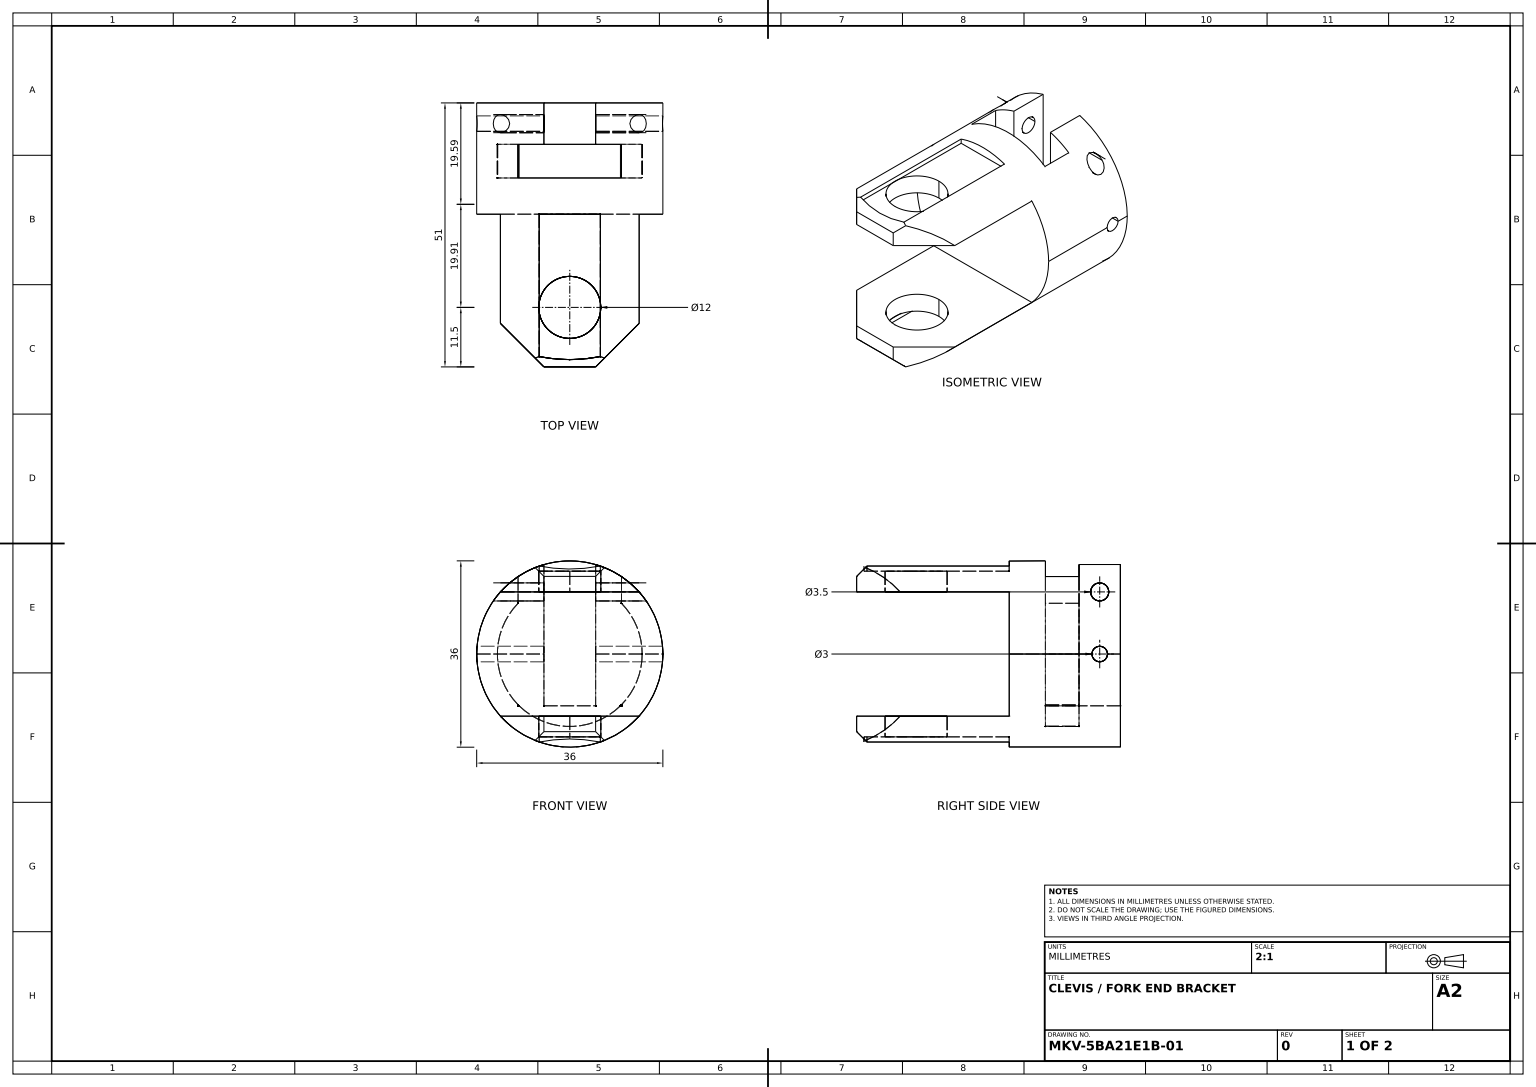
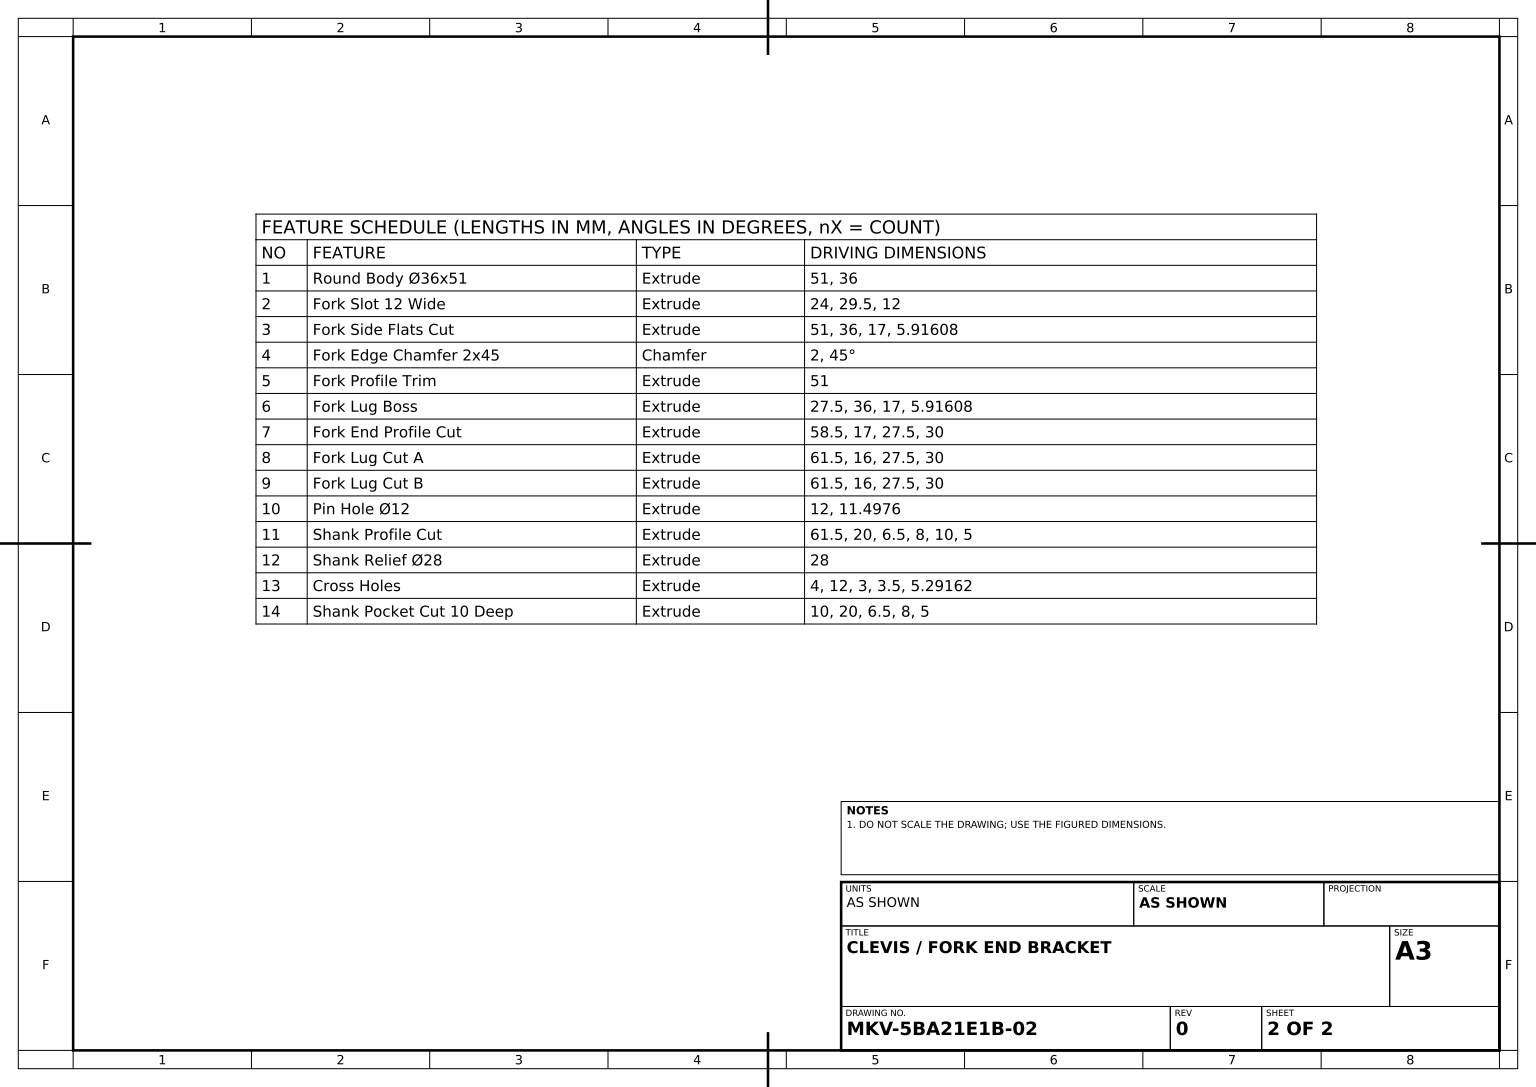
from build123d import *

# Parameters (mm, degrees)
ROUND_BODY_SKETCH_36_R         = 18
ROUND_BODY_36X51_DEPTH         = 51
FORK_SLOT_12_WIDE_DEPTH        = 58
FORK_SLOT_12_WIDE_DEPTH_BACK   = 58
FORK_SLOT_SKETCH_W             = 29.5
FORK_SLOT_SKETCH_H             = 24
FORK_SIDE_FLATS_CUT_DEPTH      = 51
FORK_EDGE_CHAMFER_2X45_SIZE    = 2
FORK_PROFILE_TRIM_DEPTH        = 25.5
FORK_LUG_BOSS_DEPTH            = 27.5
FORK_START                     = 17
FORK_END_PROFILE_SKETCH_W      = 11.832159566
FORK_END_PROFILE_SKETCH_H      = 27.5
FORK_END_PROFILE_CUT_DEPTH     = 58.5
FORK_START_2                   = -16
SKETCH9_5_W                    = 11.832159566
SKETCH9_5_H                    = 27.5
FORK_LUG_CUT_A_DEPTH           = 61.5
FORK_START_3                   = 77.5
SKETCH9_6_W                    = 11.832159566
SKETCH9_6_H                    = 27.5
FORK_LUG_CUT_B_DEPTH           = 61.5
PIN_HOLE_12_REACH              = 65.883
PIN_HOLE_SKETCH_12_R           = 6
SHANK_PROFILE_SKETCH_W         = 20
SHANK_PROFILE_SKETCH_H         = 6.5
SHANK_PROFILE_SKETCH_W_2       = 10
SHANK_PROFILE_SKETCH_H_2       = 8
SHANK_PROFILE_CUT_DEPTH        = 61.5
SHANK_RELIEF_SKETCH_28_R       = 14
SHANK_RELIEF_28_DEPTH          = 6.5
CROSS_HOLES_DEPTH              = 59.77074102
CROSS_HOLES_DEPTH_BACK         = 59.77074102
CROSS_HOLES_SKETCH_R           = 1.75
CROSS_HOLES_SKETCH_R_2         = 1.5
SKETCH11_3_W                   = 10
SKETCH11_3_H                   = 8
SKETCH11_3_W_2                 = 20
SKETCH11_3_H_2                 = 6.5
SHANK_POCKET_CUT_10_DEEP_DEPTH = 10


with BuildPart() as part:
    # Round Body Sketch _36 → Round Body _36x51 (new body)
    with BuildSketch(Plane.XY):
        Circle(ROUND_BODY_SKETCH_36_R)
    extrude(amount=ROUND_BODY_36X51_DEPTH)

    # Fork Slot Sketch → Fork Slot 12 Wide (cut, two sides: drawn at the far end of the back side and taken through both)
    with BuildSketch(Plane(origin=(0, 0, 0), x_dir=(0, 0, -1), z_dir=(1, 0, 0)).offset(-FORK_SLOT_12_WIDE_DEPTH_BACK)):
        with Locations((-36.25, 0)):
            Rectangle(FORK_SLOT_SKETCH_W, FORK_SLOT_SKETCH_H)
    extrude(amount=FORK_SLOT_12_WIDE_DEPTH + FORK_SLOT_12_WIDE_DEPTH_BACK, mode=Mode.SUBTRACT)

    # Fork Flats Sketch → Fork Side Flats Cut (cut)
    with BuildSketch(Plane.XY.offset(21.5)):
        with BuildLine():
            Line((-5.916079783, 17), (5.916079783, 17))
            ThreePointArc((5.916079783, 17), (0, 18), (-5.916079783, 17))
        make_face()
        with BuildLine():
            Line((-5.916079783, -17), (5.916079783, -17))
            ThreePointArc((5.916079783, -17), (0, -18), (-5.916079783, -17))
        make_face()
    extrude(amount=FORK_SIDE_FLATS_CUT_DEPTH, mode=Mode.SUBTRACT)

    # Fork Edge Chamfer 2x45
    fork_edge_chamfer_2x45_edges = [part.edges().sort_by_distance(p)[0] for p in [
        (0, -17, 51),
        (0, 17, 51),
    ]]
    chamfer(fork_edge_chamfer_2x45_edges, length=FORK_EDGE_CHAMFER_2X45_SIZE)

    # Fork Profile Trim Sketch → Fork Profile Trim (cut, symmetric)
    with BuildSketch(Plane(origin=(0, 0, 0), x_dir=(1, 0, 0), z_dir=(0, 1, 0))):
        Polygon((-13.416407865, -51), (-5, -51), (-13.416407865, -42.583592135), align=None)
        Polygon((13.416407865, -42.583592135), (5, -51), (13.416407865, -51), align=None)
    extrude(amount=FORK_PROFILE_TRIM_DEPTH, both=True, mode=Mode.SUBTRACT)

    # Sketch5_2 → Fork Lug Boss (add)
    with BuildSketch(Plane.XY.offset(21.5)):
        with BuildLine():
            Line((-5.916079783, 17), (5.916079783, 17))
            ThreePointArc((5.916079783, 17), (0, 18), (-5.916079783, 17))
        make_face()
        with BuildLine():
            Line((-5.916079783, -17), (5.916079783, -17))
            ThreePointArc((5.916079783, -17), (0, -18), (-5.916079783, -17))
        make_face()
    extrude(amount=FORK_LUG_BOSS_DEPTH)

    # Fork End Profile Sketch → Fork End Profile Cut (cut)
    with BuildSketch(Plane(origin=(0, 0, 0), x_dir=(1, 0, 0), z_dir=(0, 1, 0)).offset(FORK_START)):
        with BuildLine():
            Line((-5.916079783, -49), (5.916079783, -49))
            ThreePointArc((5.916079783, -49), (0, -49.58911766), (-5.916079783, -49))
        make_face()
        with Locations((0, -35.25)):
            Rectangle(FORK_END_PROFILE_SKETCH_W, FORK_END_PROFILE_SKETCH_H)
    extrude(amount=FORK_END_PROFILE_CUT_DEPTH, mode=Mode.SUBTRACT)

    # Sketch9_5 → Fork Lug Cut A (cut)
    with BuildSketch(Plane(origin=(0, 0, 0), x_dir=(1, 0, 0), z_dir=(0, 1, 0)).offset(FORK_START_2)):
        with BuildLine():
            Line((-5.916079783, -49), (5.916079783, -49))
            ThreePointArc((5.916079783, -49), (0, -49.58911766), (-5.916079783, -49))
        make_face()
        with Locations((0, -35.25)):
            Rectangle(SKETCH9_5_W, SKETCH9_5_H)
    extrude(amount=-FORK_LUG_CUT_A_DEPTH, mode=Mode.SUBTRACT)

    # Sketch9_6 → Fork Lug Cut B (cut)
    with BuildSketch(Plane(origin=(0, 0, 0), x_dir=(1, 0, 0), z_dir=(0, 1, 0)).offset(FORK_START_3)):
        with BuildLine():
            Line((-5.916079783, -49), (5.916079783, -49))
            ThreePointArc((5.916079783, -49), (0, -49.58911766), (-5.916079783, -49))
        make_face()
        with Locations((0, -35.25)):
            Rectangle(SKETCH9_6_W, SKETCH9_6_H)
    extrude(amount=-FORK_LUG_CUT_B_DEPTH, mode=Mode.SUBTRACT)

    # Pin Hole _12: up to this face of the body (flat: up to its plane)
    pin_hole_12_end = Plane(part.part.faces().sort_by_distance((0, 16, 35.447312863))[0])
    # Pin Hole Sketch _12 → Pin Hole _12 (cut, up to the picked face)
    with BuildSketch(Plane.XZ.offset(16), mode=Mode.PRIVATE) as pin_hole_12_sk1:
        with Locations(Location((0, 39.502412714, 0), (0, 0, 270))):
            Circle(PIN_HOLE_SKETCH_12_R)
    pin_hole_12_tool1 = split(extrude(pin_hole_12_sk1.sketch, amount=-PIN_HOLE_12_REACH, mode=Mode.PRIVATE), bisect_by=pin_hole_12_end, keep=Keep.BOTH, mode=Mode.PRIVATE)
    add(pin_hole_12_tool1.solids().sort_by(Axis((0, -16, 39.502413), (0, 1, 0)))[0], mode=Mode.SUBTRACT)

    # Shank Profile Sketch → Shank Profile Cut (cut)
    with BuildSketch(Plane(origin=(0, 0, 0), x_dir=(1, 0, 0), z_dir=(0, 1, 0))):
        with Locations((0, -11.25)):
            Rectangle(SHANK_PROFILE_SKETCH_W, SHANK_PROFILE_SKETCH_H)
        with Locations((0, -4)):
            Rectangle(SHANK_PROFILE_SKETCH_W_2, SHANK_PROFILE_SKETCH_H_2)
    extrude(amount=SHANK_PROFILE_CUT_DEPTH, mode=Mode.SUBTRACT)

    # Shank Relief Sketch _28 → Shank Relief _28 (cut)
    with BuildSketch(Plane(origin=(0, 0, 14.5), x_dir=(-1, 0, 0), z_dir=(0, 0, -1))):
        Circle(SHANK_RELIEF_SKETCH_28_R)
    extrude(amount=SHANK_RELIEF_28_DEPTH, mode=Mode.SUBTRACT)

    # Cross Holes Sketch → Cross Holes (cut, two sides: drawn at the far end of the back side and taken through both)
    with BuildSketch(Plane(origin=(-5, 0, 0), x_dir=(0, 0, -1), z_dir=(1, 0, 0)).offset(-CROSS_HOLES_DEPTH_BACK)):
        with Locations((-4, 12)):
            Circle(CROSS_HOLES_SKETCH_R)
        with Locations((-4, 0)):
            Circle(CROSS_HOLES_SKETCH_R_2)
    extrude(amount=CROSS_HOLES_DEPTH + CROSS_HOLES_DEPTH_BACK, mode=Mode.SUBTRACT)

    # Sketch11_3 → Shank Pocket Cut 10 Deep (cut)
    with BuildSketch(Plane(origin=(0, 0, 0), x_dir=(1, 0, 0), z_dir=(0, 1, 0))):
        with Locations((0, -4)):
            Rectangle(SKETCH11_3_W, SKETCH11_3_H)
        with Locations((0, -11.25)):
            Rectangle(SKETCH11_3_W_2, SKETCH11_3_H_2)
    extrude(amount=-SHANK_POCKET_CUT_10_DEEP_DEPTH, mode=Mode.SUBTRACT)


solid = part.part
